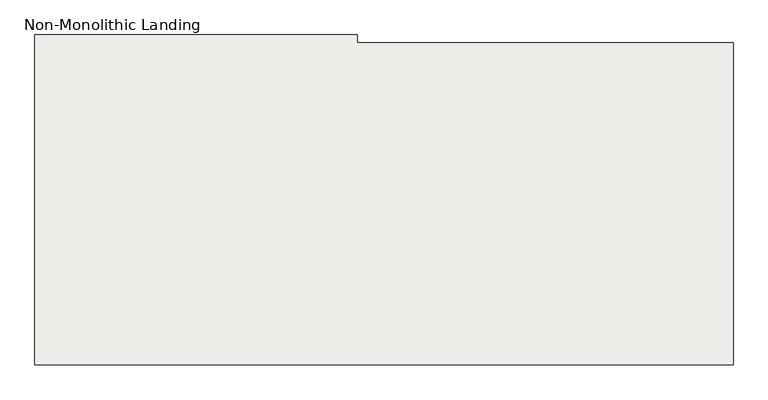
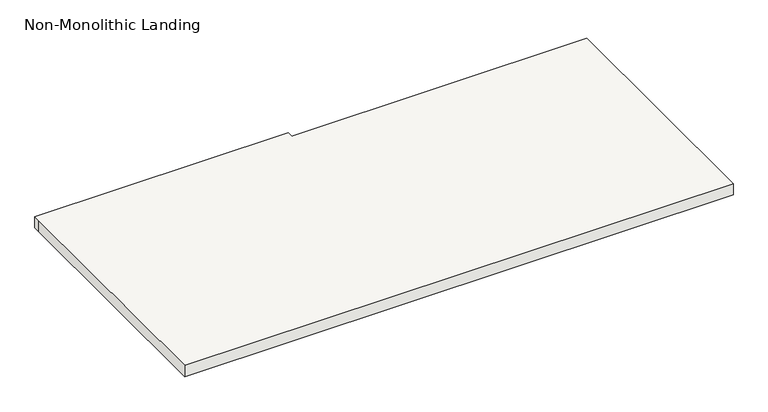
"""IFC4 building model written with IfcOpenShell, lengths in millimetres: slab geometry, Non-Monolithic Landing."""

from ifc_helpers import new_model, si_unit, origin, place, context, project, spatial, faceted_brep, source, transform, mapped, element, save


def non_monolithic_landing_175d1c90(model_context):
    return source(origin(), model_context, "Body", "Brep", [
        faceted_brep([(-15047.8847893, 9995.9922903, 4636.0772727), (-15047.8847893, 9970.5922903, 4610.6772727), (-16114.6847893, 9970.5922903, 4610.6772727), (-16114.6847893, 9995.9922903, 4636.0772727), (-16292.4847893, 9995.9922903, 4655.1272727), (-16292.4847893, 10021.3922903, 4655.1272727), (-17359.2847893, 10021.3922903, 4655.1272727), (-17359.2847893, 9995.9922903, 4655.1272727), (-17359.2847893, 8929.1922903, 4655.1272727), (-15047.8847893, 8929.1922903, 4655.1272727), (-15047.8847893, 9995.9922903, 4655.1272727), (-16114.6847893, 9970.5922903, 4604.3272727), (-15047.8847893, 9970.5922903, 4604.3272727), (-15047.8847893, 8929.1922903, 4604.3272727), (-17359.2847893, 8929.1922903, 4604.3272727), (-17359.2847893, 9995.9922903, 4604.3272727), (-17359.2847893, 10021.3922903, 4604.3272727), (-16292.4847893, 10021.3922903, 4604.3272727), (-16292.4847893, 9995.9922903, 4604.3272727), (-16114.6847893, 9995.9922903, 4604.3272727)], [[[0, 1, 2, 3]], [[4, 5, 6, 7, 8, 9, 10]], [[11, 12, 13, 14, 15, 16, 17, 18, 19]], [[12, 11, 2, 1]], [[11, 19, 3, 2]], [[4, 10, 0, 3, 19, 18]], [[5, 4, 18, 17]], [[6, 5, 17, 16]], [[7, 6, 16, 15]], [[8, 7, 15, 14]], [[9, 8, 14, 13]], [[10, 9, 13, 12, 1, 0]]]),
    ])


if __name__ == "__main__":
    model = new_model("IFC4")
    model_context = context("Model", 3, world=origin())
    ifc_project = project(units=[si_unit("LENGTHUNIT", "METRE", prefix="MILLI")], contexts=[model_context])
    site = spatial("IfcSite", under=ifc_project)
    building = spatial("IfcBuilding", under=site)
    placement = place(None, origin())
    non_monolithic_landing_shape = non_monolithic_landing_175d1c90(model_context)
    element("IfcSlab", 1, ObjectType="Non-Monolithic Landing", at=placement, inside=building, context=model_context, shape_type="MappedRepresentation", body=[
        mapped(non_monolithic_landing_shape, transform((0.0, 0.0, 0.0), x_axis=(1.0, 0.0, 0.0), y_axis=(0.0, 1.0, 0.0), z_axis=(0.0, 0.0, 1.0))),
    ])
    save(model, "model.ifc")
